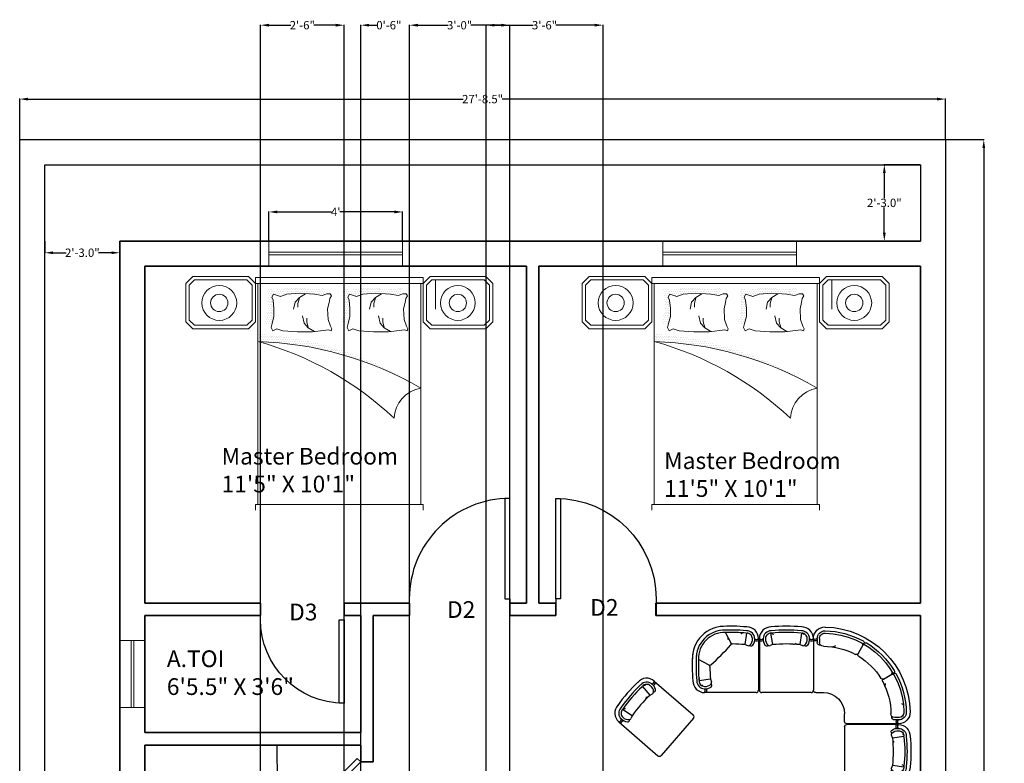
# Model space of a CAD drawing. Units: inches. Extents: x 593 to 1000, y 91 to 964.
# Tile 4 of 4: x 646 to 1000, y 697 to 964. Entities that reach past the tile are written whole.
import ezdxf

# ---------------------------------------------------------------- set-up
doc = ezdxf.new("R2010")
doc.units = ezdxf.units.IN
doc.header["$MEASUREMENT"] = 0
for name, color, linetype, lineweight in [('A-ANNO-DIMS', 2, 'Continuous', 13), ('A-ANNO-TEXT', 7, 'Continuous', 18), ('A-AREA-IDEN', 7, 'Continuous', 18), ('A-DOOR', 4, 'Continuous', 25), ('A-GLAZ', 4, 'Continuous', 18), ('A-WALL', 7, 'Continuous', 35), ('C-PROP', 7, 'Continuous', 30), ('FUR', 8, 'Continuous', 18)]:
    doc.layers.add(name, color=color, linetype=linetype, lineweight=lineweight)
doc.layers.add('ID-LOOSE', color=31, linetype='Continuous')
doc.layers.add('ID-LOOSE2', color=8, linetype='Continuous')
doc.styles.get("Standard").update_dxf_attribs({"font": 'arial.ttf'})
doc.dimstyles.get("Standard").update_dxf_attribs({"dimtxt": 3, "dimasz": 3, "dimexe": 0.18, "dimexo": 0.0625, "dimgap": 0.09, "dimtad": 0, "dimtih": 1, "dimtoh": 1, "dimdec": 1, "dimzin": 0, "dimdsep": 46, "dimlunit": 3, "dimtxsty": 'Standard', "dimcen": 0.09, "dimadec": 0, "dimazin": 0, "dimtfac": 1, "dimtdec": 1, "dimtofl": 0, "dimtmove": 0, "dimatfit": 3, "dimfxl": 1, "dimtolj": 1, "dimtzin": 0, "dimarcsym": 0})
pattern_1 = [(360, (-204.55691, -125.780183), (0.0079375, 0.015875), [0, -0.015875])]

# ---------------------------------------------------------------- blocks, each defined once
blk = doc.blocks.new('*U4')
for p, q in [((-30, 0), (-30, -6)), ((0, 0), (0, -6))]:
    blk.add_line(p, q)
blk.add_lwpolyline([(0, 0), (-21.21, 21.21), (-22.45, 19.98), (-1.24, -1.24)], close=True)
blk.add_arc((0, 0), 30, 135, 180)
blk = doc.blocks.new('*U6')
for p, q in [((-30, 0), (-30, -6)), ((0, 0), (0, -6))]:
    blk.add_line(p, q)
blk.add_lwpolyline([(0, 0), (0, 30), (-1.75, 30), (-1.75, 0)], close=True)
blk.add_arc((0, 0), 30, 90, 180)
blk = doc.blocks.new('*U5')
for p, q in [((0, 0), (0, 6)), ((36, 0), (36, 6))]:
    blk.add_line(p, q)
blk.add_lwpolyline([(0, 0), (0, -36), (1.75, -36), (1.75, 0)], close=True)
blk.add_arc((0, 0), 36, 270, 0)
blk = doc.blocks.new('A$C9d18b682')
h = blk.add_hatch()
h.set_pattern_fill('DOTS', color=256, scale=0.01, style=0)
h.set_pattern_definition(pattern_1)
h.paths.add_polyline_path([(1.2038, 1.8915), (1.1915, 1.9099), (1.1638, 1.9099), (1.1238, 1.8945), (1.0562, 1.9068), (0.927, 1.916), (0.8193, 1.9068), (0.7639, 1.8884), (0.7055, 1.9068), (0.6901, 1.8822), (0.7024, 1.8546), (0.7086, 1.7839), (0.7086, 1.7163), (0.6932, 1.6548), (0.6839, 1.621), (0.6993, 1.5933), (0.7332, 1.6087), (0.7433, 1.6057), (0.7585, 1.6664), (0.7585, 1.734), (0.7523, 1.8047), (0.74, 1.8324), (0.7554, 1.857), (0.8139, 1.8385), (0.8692, 1.857), (0.9769, 1.8662), (1.1061, 1.857), (1.1738, 1.8447), (1.1846, 1.8488), (1.1884, 1.8699)])
h.paths.add_polyline_path([(1.8571, 1.8915), (1.8448, 1.9099), (1.8171, 1.9099), (1.7771, 1.8945), (1.7095, 1.9068), (1.5803, 1.916), (1.4726, 1.9068), (1.4172, 1.8884), (1.3588, 1.9068), (1.3434, 1.8822), (1.3557, 1.8546), (1.3618, 1.7839), (1.3618, 1.7163), (1.3465, 1.6548), (1.3372, 1.621), (1.3526, 1.5933), (1.3865, 1.6087), (1.3966, 1.6057), (1.4118, 1.6664), (1.4118, 1.734), (1.4056, 1.8047), (1.3933, 1.8324), (1.4087, 1.857), (1.4672, 1.8385), (1.5225, 1.857), (1.6302, 1.8662), (1.7594, 1.857), (1.8271, 1.8447), (1.8379, 1.8488), (1.8417, 1.8699)])
h = blk.add_hatch()
h.set_pattern_fill('DOTS', color=256, scale=0.01, style=0)
h.set_pattern_definition(pattern_1)
h.paths.add_polyline_path([(0.62, 1.5186), (0.62, 1.45, -0.124273), (2.02, 1.05, 0.122563)])
for p, q in [((2.04, 2), (0.6, 2)), ((0.6, 1.95), (0.6, 2)), ((2.04, 1.95), (0.6, 1.95)), ((0.62, 0.05), (0.62, 1.95)), ((2.02, 1.95), (2.02, 0.05)), ((2.04, 2), (2.04, 1.95)), ((2.1476, 1.9789), (2.1476, 1.7289)), ((2.04, 0.05), (0.6, 0.05)), ((0.6, 0), (0.6, 0.05)), ((2.04, 0.05), (2.04, 0))]:
    blk.add_line(p, q)
for points in [[(0.06, 1.56), (0.54, 1.56), (0.6, 1.62), (0.6, 1.95), (0.54, 2.01), (0.06, 2.01), (0, 1.95), (0, 1.62)], [(0.075, 1.59), (0.525, 1.59), (0.57, 1.635), (0.57, 1.935), (0.525, 1.98), (0.075, 1.98), (0.03, 1.935), (0.03, 1.635)], [(2.1, 1.56), (2.58, 1.56), (2.64, 1.62), (2.64, 1.95), (2.58, 2.01), (2.1, 2.01), (2.04, 1.95), (2.04, 1.62)], [(2.115, 1.59), (2.565, 1.59), (2.61, 1.635), (2.61, 1.935), (2.565, 1.98), (2.115, 1.98), (2.07, 1.935), (2.07, 1.635)]]:
    blk.add_lwpolyline(points, close=True)
for points in [[(0.8139, 1.8385), (0.7554, 1.857), (0.74, 1.8324), (0.7523, 1.8047), (0.7585, 1.734), (0.7585, 1.6664), (0.7431, 1.6049), (0.7339, 1.5711), (0.7493, 1.5434), (0.7831, 1.5588), (0.8354, 1.5434), (0.9615, 1.5342), (1.0907, 1.5342), (1.2261, 1.5496), (1.2507, 1.5434), (1.2568, 1.5588), (1.2445, 1.5834), (1.223, 1.6387), (1.2199, 1.7309), (1.2322, 1.7863), (1.2384, 1.8201), (1.2538, 1.8416), (1.2414, 1.86), (1.2138, 1.86), (1.1738, 1.8447), (1.1061, 1.857), (0.9769, 1.8662), (0.8692, 1.857), (0.8139, 1.8385)], [(1.4672, 1.8385), (1.4087, 1.857), (1.3933, 1.8324), (1.4056, 1.8047), (1.4118, 1.734), (1.4118, 1.6664), (1.3964, 1.6049), (1.3872, 1.5711), (1.4026, 1.5434), (1.4364, 1.5588), (1.4887, 1.5434), (1.6148, 1.5342), (1.744, 1.5342), (1.8794, 1.5496), (1.904, 1.5434), (1.9101, 1.5588), (1.8978, 1.5834), (1.8763, 1.6387), (1.8732, 1.7309), (1.8855, 1.7863), (1.8917, 1.8201), (1.907, 1.8416), (1.8947, 1.86), (1.8671, 1.86), (1.8271, 1.8447), (1.7594, 1.857), (1.6302, 1.8662), (1.5225, 1.857), (1.4672, 1.8385)], [(1.0292, 1.86), (0.9769, 1.8293), (0.94, 1.7893), (0.9277, 1.7279)], [(0.9769, 1.8262), (0.9646, 1.777), (0.9646, 1.7463)], [(1.6825, 1.86), (1.6302, 1.8293), (1.5933, 1.7893), (1.581, 1.7279)], [(1.6302, 1.8262), (1.6179, 1.777), (1.6179, 1.7463)], [(1.1061, 1.5373), (1.0538, 1.568), (1.0169, 1.608), (1.0046, 1.6695)], [(1.0538, 1.5711), (1.0415, 1.6203), (1.0415, 1.651)], [(1.7594, 1.5373), (1.7071, 1.568), (1.6702, 1.608), (1.6579, 1.6695)], [(1.7071, 1.5711), (1.6948, 1.6203), (1.6948, 1.651)]]:
    blk.add_lwpolyline(points)
for centre, radius in [((0.288, 1.782), 0.15), ((2.3392, 1.782), 0.15), ((0.288, 1.782), 0.0743), ((2.3392, 1.782), 0.0743)]:
    blk.add_circle(centre, radius)
for centre, radius, start, end in [((0.5277, -1.5229), 2.9743, 59.8866, 88.22261), ((-0.1045, -1.2025), 2.7497, 46.43667, 74.72336), ((2.0704, 0.7742), 0.2804, 100.35432, 176.78617)]:
    blk.add_arc(centre, radius, start, end)
blk = doc.blocks.new('A$C68294616')
at = {"layer": 'ID-LOOSE'}
for p, q in [((0.402, 0.39), (1.042, 0.39)), ((0.372, -0.31), (0.372, 0.36)), ((1.072, -0.31), (1.072, 0.36)), ((0.545, -0.231), (0.511, -0.219)), ((0.899, -0.231), (0.933, -0.219))]:
    blk.add_line(p, q, dxfattribs=at)
for centre, radius, start, end in [((0.402, 0.36), 0.03, 90, 180), ((1.042, 0.36), 0.03, 360, 90), ((0.554, -0.3), 0.133, 146.0897, 185.6132), ((0.465, -0.24), 0.025, 62.9608, 146.0897), ((0.452, -0.265), 0.0532, 51.0017, 62.9608), ((0.502, -0.242), 0.025, 70, 132.0066), ((0.722, 1.538), 1.778, 264.2835, 275.7165), ((0.628, -0.286), 0.0481, 90.6237, 136.1803), ((0.942, -0.242), 0.025, 47.9934, 110), ((0.992, -0.265), 0.0532, 117.0392, 128.9983), ((0.979, -0.24), 0.025, 33.9103, 117.0392), ((0.89, -0.3), 0.133, 354.3868, 33.9103), ((0.397, -0.346), 0.0662, 67.8298, 112.1702), ((0.522, -0.31), 0.15, 180, 271.1754), ((0.522, -0.31), 0.1, 180, 271.1754), ((0.529, -0.332), 0.0481, 216.0775, 261.6341), ((0.933, -0.336), 0.0481, 201.2156, 246.7721), ((0.922, -0.31), 0.15, 268.8246, 360), ((0.922, -0.31), 0.1, 268.8246, 360), ((1.047, -0.346), 0.0662, 67.8298, 112.1702), ((0.722, 1.538), 2.008, 264.2835, 275.7165), ((0.722, 1.538), 1.958, 264.2835, 275.7165)]:
    blk.add_arc(centre, radius, start, end, dxfattribs=at)
at = {"layer": 'ID-LOOSE2'}
for p, q in [((0.545, -0.231), (0.522, -0.38)), ((0.899, -0.231), (0.922, -0.38))]:
    blk.add_line(p, q, dxfattribs=at)
for centre, radius, start, end in [((0.554, -0.3), 0.103, 132.0066, 185.6132), ((0.89, -0.3), 0.103, 354.3868, 47.9934), ((0.397, -0.336), 0.0362, 46.3972, 133.6028), ((0.522, -0.31), 0.07, 180, 271.1754), ((0.722, 1.538), 1.928, 264.2835, 275.7165), ((0.922, -0.31), 0.07, 268.8246, 360), ((1.047, -0.336), 0.0362, 46.3972, 133.6028)]:
    blk.add_arc(centre, radius, start, end, dxfattribs=at)
blk = doc.blocks.new('A$C707258B2')
at = {"layer": 'ID-LOOSE'}
for p, q in [((0.404, 0.342), (1.074, 0.342)), ((0.404, 0.292), (0.454, 0.292)), ((1.104, 0.312), (1.104, 0.212)), ((1.479, -0.063), (1.379, -0.063)), ((1.509, -0.763), (1.509, -0.093)), ((1.459, -0.763), (1.459, -0.712))]:
    blk.add_line(p, q, dxfattribs=at)
for centre, radius, start, end in [((0.404, 0.192), 0.15, 90, 181.1754), ((0.404, 0.192), 0.1, 90, 181.1754), ((0.368, 0.317), 0.0662, 337.8298, 22.1702), ((0.455, 0.256), 0.0357, 345.4262, 90.5555), ((0.454, 0.212), 0.05, 360, 90), ((1.074, 0.312), 0.03, 360, 90), ((1.379, 0.212), 1.125, 181.1754, 268.8246), ((1.379, 0.212), 1.075, 181.1754, 208.6357), ((1.379, 0.212), 0.875, 180, 208.4082), ((1.379, 0.212), 0.275, 180, 270), ((0.419, 0.102), 0.0935, 329.1864, 354.4231), ((1.479, -0.093), 0.03, 360, 90), ((0.587, -0.216), 0.025, 300, 28.4082), ((0.612, -0.259), 0.025, 31.5918, 120), ((1.379, 0.212), 0.875, 211.5918, 238.4082), ((0.457, -0.291), 0.025, 208.6357, 300), ((0.482, -0.334), 0.025, 120, 211.3643), ((1.379, 0.212), 1.075, 211.3643, 238.6357), ((0.461, -0.295), 0.0199, 309.2667, 10.0983), ((0.481, -0.329), 0.0199, 49.9017, 110.7333), ((0.907, -0.555), 0.025, 330, 58.4082), ((0.951, -0.58), 0.025, 61.5918, 150), ((1.379, 0.212), 0.875, 241.5918, 270), ((1.019, -0.683), 0.0935, 84.0982, 109.3349), ((0.832, -0.685), 0.025, 238.6357, 330), ((0.876, -0.71), 0.025, 150, 241.3643), ((0.838, -0.686), 0.0199, 339.2667, 40.0983), ((0.872, -0.706), 0.0199, 79.9017, 140.7333), ((1.379, 0.212), 1.075, 241.3643, 268.8246), ((1.359, -0.763), 0.15, 268.8246, 360), ((1.359, -0.763), 0.1, 268.8246, 360), ((1.379, -0.713), 0.05, 360, 90), ((1.425, -0.709), 0.0336, 354.6301, 109.3883), ((1.484, -0.799), 0.0662, 67.8298, 112.1702), ((1.291, -0.783), 0.0481, 201.2156, 246.7721), ((1.405, -0.803), 0.00999, 211.067, 288.5313)]:
    blk.add_arc(centre, radius, start, end, dxfattribs=at)
at = {"layer": 'ID-LOOSE2'}
for p, q in [((0.404, 0.262), (0.454, 0.262)), ((0.6, -0.238), (0.47, -0.313)), ((0.929, -0.567), (0.854, -0.697)), ((1.429, -0.763), (1.429, -0.713))]:
    blk.add_line(p, q, dxfattribs=at)
for centre, radius, start, end in [((0.404, 0.192), 0.07, 90, 181.1754), ((0.378, 0.317), 0.0362, 316.3972, 43.6028), ((1.379, 0.212), 1.045, 181.1754, 268.8246), ((1.359, -0.763), 0.07, 268.8246, 360), ((1.484, -0.789), 0.0362, 46.3972, 133.6028)]:
    blk.add_arc(centre, radius, start, end, dxfattribs=at)
blk = doc.blocks.new('A$C68FE3AF0')
at = {"layer": 'ID-LOOSE'}
for p, q in [((0.402, 0.39), (1.072, 0.39)), ((0.372, -0.31), (0.372, 0.36)), ((0.993, 0.217), (0.981, 0.251)), ((0.545, -0.231), (0.511, -0.219))]:
    blk.add_line(p, q, dxfattribs=at)
for centre, radius, start, end in [((0.402, 0.36), 0.03, 90, 180), ((1.098, 0.365), 0.0562, 153.6122, 206.6666), ((1.072, 0.24), 0.15, 358.8246, 90), ((1.002, 0.297), 0.025, 123.9103, 207.0392), ((1.004, 0.26), 0.025, 137.9934, 200), ((1.027, 0.31), 0.0532, 207.0392, 218.9983), ((1.062, 0.208), 0.133, 84.3868, 123.9103), ((1.072, 0.24), 0.1, 358.8246, 90), ((1.111, 0.29), 0.0136, 109.4209, 182.5668), ((-0.776, 0.04), 1.778, 0.3836, 5.7165), ((1.121, 0.22), 0.0246, 302.8172, 29.8385), ((-0.776, 0.04), 1.958, 355.8657, 5.7165), ((-0.776, 0.04), 2.008, 355.818, 5.7165), ((2.592, -1.83), 2.454, 130.6961, 139.3039), ((1.005, 0.016), 0.02, 62, 130.6961), ((1.022, 0.052), 0.02, 180.3836, 242), ((0.812, -0.05), 0.419, 268.2181, 1.7819), ((0.812, -0.05), 0.369, 268.2181, 1.7819), ((0.554, -0.3), 0.133, 146.0897, 185.6132), ((0.465, -0.24), 0.025, 62.9608, 146.0897), ((0.452, -0.265), 0.0532, 51.0017, 62.9608), ((0.502, -0.242), 0.025, 70, 132.0066), ((0.722, 1.538), 1.778, 264.2835, 269.6164), ((0.71, -0.26), 0.02, 28, 89.6164), ((0.746, -0.243), 0.02, 139.3039, 208), ((0.397, -0.336), 0.0562, 63.3334, 116.3878), ((0.522, -0.31), 0.15, 180, 271.1754), ((0.522, -0.31), 0.1, 180, 271.1754), ((0.575, -0.358), 0.0246, 281.4741, 324.9847), ((0.581, -0.359), 0.0246, 281.4741, 324.9847), ((0.786, -0.309), 0.0246, 151.3726, 194.8832), ((0.788, -0.313), 0.0246, 151.3726, 194.8832), ((0.722, 1.538), 2.008, 264.2835, 274.182), ((0.722, 1.538), 1.958, 264.2835, 274.1343)]:
    blk.add_arc(centre, radius, start, end, dxfattribs=at)
at = {"layer": 'ID-LOOSE2'}
for p, q in [((0.993, 0.217), (1.142, 0.24)), ((1.013, 0.034), (1.15, -0.039)), ((0.545, -0.231), (0.522, -0.38)), ((0.728, -0.251), (0.801, -0.388))]:
    blk.add_line(p, q, dxfattribs=at)
for centre, radius, start, end in [((1.098, 0.365), 0.0362, 136.3972, 223.6028), ((1.062, 0.208), 0.103, 84.3868, 137.9934), ((1.072, 0.24), 0.07, 358.8246, 90), ((-0.776, 0.04), 1.928, 357.6546, 5.7165), ((0.812, -0.05), 0.339, 268.2181, 1.7819), ((0.554, -0.3), 0.103, 132.0066, 185.6132), ((0.397, -0.336), 0.0362, 46.3972, 133.6028), ((0.522, -0.31), 0.07, 180, 271.1754), ((0.722, 1.538), 1.928, 264.2835, 272.3454)]:
    blk.add_arc(centre, radius, start, end, dxfattribs=at)
blk = doc.blocks.new('*D25')
at = {"layer": 'A-ANNO-DIMS', "color": 0, "lineweight": -2, "transparency": 16777216}
for p, q in [((654.91, 884.22), (654.91, 879.89)), ((681.91, 884.22), (681.91, 879.89)), ((657.91, 880.07), (662.56, 880.07)), ((678.91, 880.07), (674.26, 880.07))]:
    blk.add_line(p, q, dxfattribs=at)
at = {"layer": 'A-ANNO-DIMS', "color": 0, "transparency": 16777216}
for points in [[(657.91, 880.57), (657.91, 879.57), (654.91, 880.07)], [(678.91, 880.57), (678.91, 879.57), (681.91, 880.07)]]:
    blk.add_solid(points, dxfattribs=at)
at = {"layer": 'Defpoints', "color": 0, "transparency": 16777216}
for p in [(654.91, 884.28), (681.91, 884.28), (654.91, 880.07)]:
    blk.add_point(p, dxfattribs=at)
at = {"layer": 'A-ANNO-DIMS', "color": 0, "transparency": 16777216, "insert": (668.41, 880.07), "char_height": 3, "attachment_point": 5}
blk.add_mtext('\\A1;2\'-3.0"', dxfattribs=at)
blk = doc.blocks.new('*D26')
at = {"layer": 'A-ANNO-DIMS', "color": 0, "lineweight": -2, "transparency": 16777216}
for p, q in [((969.35, 911.68), (956.26, 911.68)), ((956.44, 908.68), (956.44, 899.61)), ((956.44, 887.28), (956.44, 896.36)), ((969.35, 884.28), (956.26, 884.28))]:
    blk.add_line(p, q, dxfattribs=at)
at = {"layer": 'A-ANNO-DIMS', "color": 0, "transparency": 16777216}
for points in [[(955.94, 908.68), (956.94, 908.68), (956.44, 911.68)], [(955.94, 887.28), (956.94, 887.28), (956.44, 884.28)]]:
    blk.add_solid(points, dxfattribs=at)
at = {"layer": 'Defpoints', "color": 0, "transparency": 16777216}
for p in [(956.44, 911.68), (969.41, 911.68), (969.41, 884.28)]:
    blk.add_point(p, dxfattribs=at)
at = {"layer": 'A-ANNO-DIMS', "color": 0, "transparency": 16777216, "insert": (956.44, 897.98), "char_height": 3, "attachment_point": 5}
blk.add_mtext('\\A1;2\'-3.0"', dxfattribs=at)
blk = doc.blocks.new('*D27')
at = {"layer": 'A-ANNO-DIMS', "color": 0, "lineweight": -2, "transparency": 16777216}
for p, q in [((735.41, 884.35), (735.41, 894.9)), ((738.41, 894.72), (757.88, 894.72)), ((780.41, 894.72), (760.94, 894.72)), ((783.41, 884.35), (783.41, 894.9))]:
    blk.add_line(p, q, dxfattribs=at)
at = {"layer": 'A-ANNO-DIMS', "color": 0, "transparency": 16777216}
for points in [[(738.41, 895.22), (738.41, 894.22), (735.41, 894.72)], [(780.41, 895.22), (780.41, 894.22), (783.41, 894.72)]]:
    blk.add_solid(points, dxfattribs=at)
at = {"layer": 'Defpoints', "color": 0, "transparency": 16777216}
for p in [(783.41, 894.72), (735.41, 884.28), (783.41, 884.28)]:
    blk.add_point(p, dxfattribs=at)
at = {"layer": 'A-ANNO-DIMS', "color": 0, "transparency": 16777216, "insert": (759.41, 894.72), "char_height": 3, "attachment_point": 5}
blk.add_mtext("\\A1;4'", dxfattribs=at)
blk = doc.blocks.new('*D29')
at = {"layer": 'A-ANNO-DIMS', "color": 0, "lineweight": -2, "transparency": 16777216}
for p, q in [((978.47, 920.68), (992.35, 920.68)), ((992.17, 917.68), (992.17, 530.06)), ((992.17, 139.18), (992.17, 526.81)), ((978.47, 136.18), (992.35, 136.18))]:
    blk.add_line(p, q, dxfattribs=at)
at = {"layer": 'A-ANNO-DIMS', "color": 0, "transparency": 16777216}
for points in [[(991.67, 917.68), (992.67, 917.68), (992.17, 920.68)], [(991.67, 139.18), (992.67, 139.18), (992.17, 136.18)]]:
    blk.add_solid(points, dxfattribs=at)
at = {"layer": 'Defpoints', "color": 0, "transparency": 16777216}
for p in [(978.41, 920.68), (992.17, 920.68), (978.41, 136.18)]:
    blk.add_point(p, dxfattribs=at)
at = {"layer": 'A-ANNO-DIMS', "color": 0, "transparency": 16777216, "insert": (992.17, 528.43), "char_height": 3, "attachment_point": 5}
blk.add_mtext('\\A1;65\'-4.5"', dxfattribs=at)
blk = doc.blocks.new('*D30')
at = {"layer": 'A-ANNO-DIMS', "color": 0, "lineweight": -2, "transparency": 16777216}
for p, q in [((645.91, 920.75), (645.91, 935.42)), ((648.91, 935.24), (805.14, 935.24)), ((975.41, 935.24), (819.18, 935.24)), ((978.41, 920.75), (978.41, 935.42))]:
    blk.add_line(p, q, dxfattribs=at)
at = {"layer": 'A-ANNO-DIMS', "color": 0, "transparency": 16777216}
for points in [[(648.91, 935.74), (648.91, 934.74), (645.91, 935.24)], [(975.41, 935.74), (975.41, 934.74), (978.41, 935.24)]]:
    blk.add_solid(points, dxfattribs=at)
at = {"layer": 'Defpoints', "color": 0, "transparency": 16777216}
for p in [(978.41, 935.24), (645.91, 920.68), (978.41, 920.68)]:
    blk.add_point(p, dxfattribs=at)
at = {"layer": 'A-ANNO-DIMS', "color": 0, "transparency": 16777216, "insert": (812.16, 935.24), "char_height": 3, "attachment_point": 5}
blk.add_mtext('\\A1;27\'-8.5"', dxfattribs=at)
blk = doc.blocks.new('WIN-24')
for p, q in [((9, 24), (0, 24)), ((4, 24), (4, 0)), ((5, 24), (5, 0)), ((9, 0), (0, 0))]:
    blk.add_line(p, q)
blk = doc.blocks.new('WIN-48')
for p, q in [((0, 0), (0, 9)), ((48, 0), (48, 9)), ((0, 5), (48, 5)), ((0, 4), (48, 4))]:
    blk.add_line(p, q)
blk = doc.blocks.new('*D59')
at = {"layer": 'A-ANNO-DIMS', "color": 0, "lineweight": -2, "transparency": 16777216}
for p, q in [((813.41, 441.75), (813.41, 961.96)), ((855.41, 441.75), (855.41, 961.96)), ((816.41, 961.78), (830.33, 961.78)), ((852.41, 961.78), (838.49, 961.78))]:
    blk.add_line(p, q, dxfattribs=at)
at = {"layer": 'A-ANNO-DIMS', "color": 0, "transparency": 16777216}
for points in [[(816.41, 962.28), (816.41, 961.28), (813.41, 961.78)], [(852.41, 962.28), (852.41, 961.28), (855.41, 961.78)]]:
    blk.add_solid(points, dxfattribs=at)
at = {"layer": 'Defpoints', "color": 0, "transparency": 16777216}
for p in [(855.41, 961.78), (813.41, 441.68), (855.41, 441.68)]:
    blk.add_point(p, dxfattribs=at)
at = {"layer": 'A-ANNO-DIMS', "color": 0, "transparency": 16777216, "insert": (834.41, 961.78), "char_height": 3, "attachment_point": 5}
blk.add_mtext('\\A1;3\'-6"', dxfattribs=at)
blk = doc.blocks.new('*D60')
at = {"layer": 'A-ANNO-DIMS', "color": 0, "lineweight": -2, "transparency": 16777216}
for p, q in [((785.91, 306.75), (785.91, 961.96)), ((821.91, 306.75), (821.91, 961.96)), ((788.91, 961.78), (799.83, 961.78)), ((818.91, 961.78), (807.99, 961.78))]:
    blk.add_line(p, q, dxfattribs=at)
at = {"layer": 'A-ANNO-DIMS', "color": 0, "transparency": 16777216}
for points in [[(788.91, 962.28), (788.91, 961.28), (785.91, 961.78)], [(818.91, 962.28), (818.91, 961.28), (821.91, 961.78)]]:
    blk.add_solid(points, dxfattribs=at)
at = {"layer": 'Defpoints', "color": 0, "transparency": 16777216}
for p in [(821.91, 961.78), (785.91, 306.68), (821.91, 306.68)]:
    blk.add_point(p, dxfattribs=at)
at = {"layer": 'A-ANNO-DIMS', "color": 0, "transparency": 16777216, "insert": (803.91, 961.78), "char_height": 3, "attachment_point": 5}
blk.add_mtext('\\A1;3\'-0"', dxfattribs=at)
blk = doc.blocks.new('*D61')
at = {"layer": 'A-ANNO-DIMS', "color": 0, "lineweight": -2, "transparency": 16777216}
for p, q in [((732.41, 306.75), (732.41, 961.96)), ((762.41, 306.75), (762.41, 961.96)), ((735.41, 961.78), (743.31, 961.78)), ((759.41, 961.78), (751.51, 961.78))]:
    blk.add_line(p, q, dxfattribs=at)
at = {"layer": 'A-ANNO-DIMS', "color": 0, "transparency": 16777216}
for points in [[(735.41, 962.28), (735.41, 961.28), (732.41, 961.78)], [(759.41, 962.28), (759.41, 961.28), (762.41, 961.78)]]:
    blk.add_solid(points, dxfattribs=at)
at = {"layer": 'Defpoints', "color": 0, "transparency": 16777216}
for p in [(762.41, 961.78), (732.41, 306.68), (762.41, 306.68)]:
    blk.add_point(p, dxfattribs=at)
at = {"layer": 'A-ANNO-DIMS', "color": 0, "transparency": 16777216, "insert": (747.41, 961.78), "char_height": 3, "attachment_point": 5}
blk.add_mtext('\\A1;2\'-6"', dxfattribs=at)
blk = doc.blocks.new('*D64')
at = {"layer": 'A-ANNO-DIMS', "color": 0, "lineweight": -2, "transparency": 16777216}
for p, q in [((762.41, 306.75), (762.41, 961.96)), ((768.41, 306.75), (768.41, 961.96)), ((759.41, 961.78), (756.41, 961.78)), ((771.41, 961.78), (774.41, 961.78))]:
    blk.add_line(p, q, dxfattribs=at)
at = {"layer": 'A-ANNO-DIMS', "color": 0, "transparency": 16777216}
for points in [[(759.41, 962.28), (759.41, 961.28), (762.41, 961.78)], [(771.41, 962.28), (771.41, 961.28), (768.41, 961.78)]]:
    blk.add_solid(points, dxfattribs=at)
at = {"layer": 'Defpoints', "color": 0, "transparency": 16777216}
for p in [(768.41, 961.78), (762.41, 306.68), (768.41, 306.68)]:
    blk.add_point(p, dxfattribs=at)
at = {"layer": 'A-ANNO-DIMS', "color": 0, "transparency": 16777216, "insert": (778.49, 961.78), "char_height": 3, "attachment_point": 5}
blk.add_mtext('\\A1;0\'-6"', dxfattribs=at)

msp = doc.modelspace()

# ---------------------------------------------------------------- linework, layer by layer
at = {"layer": 'A-WALL'}
for p, q in [((969.41, 884.28), (681.91, 884.28)), ((681.91, 884.28), (681.91, 528.23)), ((827.91, 875.28), (690.91, 875.28)), ((690.91, 875.28), (690.91, 754.28)), ((969.41, 875.28), (832.41, 875.28)), ((732.41, 754.28), (690.91, 754.28)), ((732.41, 749.78), (732.41, 754.28)), ((785.91, 754.28), (762.41, 754.28)), ((762.41, 749.78), (762.41, 754.28)), ((785.91, 754.28), (785.91, 749.78)), ((827.91, 754.28), (821.91, 754.28)), ((821.91, 754.28), (821.91, 749.78)), ((838.41, 754.28), (832.41, 754.28)), ((838.41, 754.28), (838.41, 749.78)), ((969.41, 754.28), (874.41, 754.28)), ((874.41, 754.28), (874.41, 749.78)), ((732.41, 749.78), (690.91, 749.78)), ((690.91, 749.78), (690.91, 707.78)), ((768.41, 749.78), (762.41, 749.78)), ((768.41, 749.78), (768.41, 707.78)), ((785.91, 749.78), (772.91, 749.78)), ((772.91, 749.78), (772.91, 703.28)), ((838.41, 749.78), (821.91, 749.78)), ((969.41, 749.78), (874.41, 749.78)), ((768.41, 707.78), (690.91, 707.78)), ((768.41, 703.28), (690.91, 703.28)), ((690.91, 703.28), (690.91, 661.28)), ((768.41, 703.28), (768.41, 697.28)), ((772.91, 703.28), (772.91, 697.28)), ((768.41, 697.28), (772.91, 697.28))]:
    msp.add_line(p, q, dxfattribs=at)
for points in [[(827.91, 754.28), (827.91, 875.28)], [(832.41, 754.28), (832.41, 875.28)], [(969.41, 875.28), (969.41, 754.28)], [(969.41, 749.78), (969.41, 614.78)]]:
    msp.add_lwpolyline(points, dxfattribs=at)
at = {"layer": 'C-PROP'}
msp.add_line((978.41, 920.68), (978.41, 136.18), dxfattribs=at)
for points in [[(678.91, 136.18), (645.91, 136.18), (645.91, 920.68), (978.41, 920.68), (978.41, 136.18), (945.41, 136.18)], [(678.91, 145.18), (654.91, 145.18), (654.91, 911.68), (969.41, 911.68), (969.41, 884.28)]]:
    msp.add_lwpolyline(points, dxfattribs=at)

# ---------------------------------------------------------------- block references
at = {"layer": 'A-DOOR', "yscale": 1.001918595307477, "zscale": 1.001918595307477, "rotation": 180}
for p, xscale in [((821.91, 755.8), 1.001918595307477), ((838.41, 755.8), -1.001918595307477)]:
    msp.add_blockref('*U5', p, dxfattribs=dict(at, xscale=xscale))
at = {"layer": 'A-DOOR', "xscale": -1, "rotation": 180}
for name, p in [('*U6', (762.41, 748.28)), ('*U4', (768.41, 697.28))]:
    msp.add_blockref(name, p, dxfattribs=at)
at = {"layer": 'A-GLAZ', "rotation": 180}
msp.add_blockref('WIN-48', (783.41, 884.28), dxfattribs=at)
at = {"layer": 'A-GLAZ'}
for name, p in [('WIN-48', (876.91, 875.28)), ('WIN-24', (681.91, 716.78))]:
    msp.add_blockref(name, p, dxfattribs=at)
at = {"layer": 'FUR', "xscale": 41.77713228862137, "yscale": 41.77713228862137, "zscale": 41.77713228862137}
for p in [(705.55, 787.61), (847.91, 787.61)]:
    msp.add_blockref('A$C9d18b682', p, dxfattribs=at)
at = {"layer": 'FUR', "yscale": 27.69884856456519, "zscale": 27.69884856456519}
for name, p, xscale, rotation in [('A$C68FE3AF0', (921.56, 732.94), 27.69884856456519, 180), ('A$C68294616', (941.26, 732.94), 27.69884856456519, 180), ('A$C707258B2', (940.43, 752.72), -27.69884856456519, 89.99999999933821), ('A$C68294616', (887.06, 728.42), 27.69884856456519, 228.9999999993411), ('A$C68294616', (952.97, 720.96), -27.69884856456519, 89.99999999933821)]:
    msp.add_blockref(name, p, dxfattribs=dict(at, xscale=xscale, rotation=rotation))

# ---------------------------------------------------------------- texts
at = {"layer": 'A-ANNO-TEXT', "char_height": 6, "attachment_point": 1}
for s, insert in [('{D3}', (742.67, 754.06)), ('{D2}', (799.37, 754.95)), ('{D2}', (850.8, 755.7))]:
    msp.add_mtext_dynamic_manual_height_columns(s, width=8.544, gutter_width=1, heights=[0], dxfattribs=dict(at, insert=insert))
at = {"layer": 'A-AREA-IDEN', "char_height": 6, "attachment_point": 1}
for s, insert in [('Master Bedroom\\P11\'5" X 10\'1"', (718.43, 810.01)), ('Master Bedroom\\P11\'5" X 10\'1"', (877.37, 808.41)), ('A.TOI\\P6\'5.5" X 3\'6"', (698.76, 737.28))]:
    msp.add_mtext_dynamic_manual_height_columns(s, width=76.3054, gutter_width=1, heights=[0], dxfattribs=dict(at, insert=insert))

# ---------------------------------------------------------------- dimensions: what is measured, and where the dimension line sits
at = {"layer": 'A-ANNO-DIMS'}
for base, p1, p2, override, picture, middle in [((762.41, 961.78), (732.41, 306.68), (762.41, 306.68), {"dimdec": 1, "dimlfac": 1, "dimrnd": 0, "dimzin": 1, "dimdsep": 46, "dimlunit": 4, "dimfrac": 2}, '*D61', (747.41, 961.78)), ((768.41, 961.78), (762.41, 306.68), (768.41, 306.68), {"dimdec": 1, "dimlfac": 1, "dimrnd": 0, "dimzin": 1, "dimdsep": 46, "dimlunit": 4, "dimfrac": 2}, '*D64', (778.49, 961.78)), ((821.91, 961.78), (785.91, 306.68), (821.91, 306.68), {"dimdec": 1, "dimlfac": 1, "dimrnd": 0, "dimzin": 1, "dimdsep": 46, "dimlunit": 4, "dimfrac": 2}, '*D60', (803.91, 961.78)), ((855.41, 961.78), (813.41, 441.68), (855.41, 441.68), {"dimdec": 1, "dimlfac": 1, "dimrnd": 0, "dimzin": 1, "dimdsep": 46, "dimlunit": 4, "dimfrac": 2}, '*D59', (834.41, 961.78)), ((978.41, 935.24), (645.91, 920.68), (978.41, 920.68), {"dimclrd": 0, "dimclre": 0, "dimclrt": 0}, '*D30', (812.16, 935.24)), ((783.41, 894.72), (735.41, 884.28), (783.41, 884.28), {"dimclrd": 0, "dimclre": 0, "dimclrt": 0}, '*D27', (759.41, 894.72)), ((654.91, 880.07), (681.91, 884.28), (654.91, 884.28), {"dimclrd": 0, "dimclre": 0, "dimclrt": 0}, '*D25', (668.41, 880.07))]:
    dim = msp.add_linear_dim(base=base, p1=p1, p2=p2, dimstyle='Standard', override=override, dxfattribs=at)
    dim.commit()
    dim.dimension.update_dxf_attribs({"geometry": picture, "text_midpoint": middle})
dim = msp.add_linear_dim(base=(992.17, 920.68), p1=(978.41, 136.18), p2=(978.41, 920.68), angle=90, dimstyle='Standard', override={"dimclrd": 0, "dimclre": 0, "dimclrt": 0}, dxfattribs=at)
dim.commit()
dim.dimension.update_dxf_attribs({"geometry": '*D29', "text_midpoint": (992.17, 528.43)})
dim = msp.add_linear_dim(base=(956.44, 911.68), p1=(969.41, 884.28), p2=(969.41, 911.68), angle=90, text='2\'-3.0"', dimstyle='Standard', override={"dimclrd": 0, "dimclre": 0, "dimclrt": 0}, dxfattribs=at)
dim.commit()
dim.dimension.update_dxf_attribs({"geometry": '*D26', "text_midpoint": (956.44, 897.98)})

doc.saveas('drawing.dxf')
